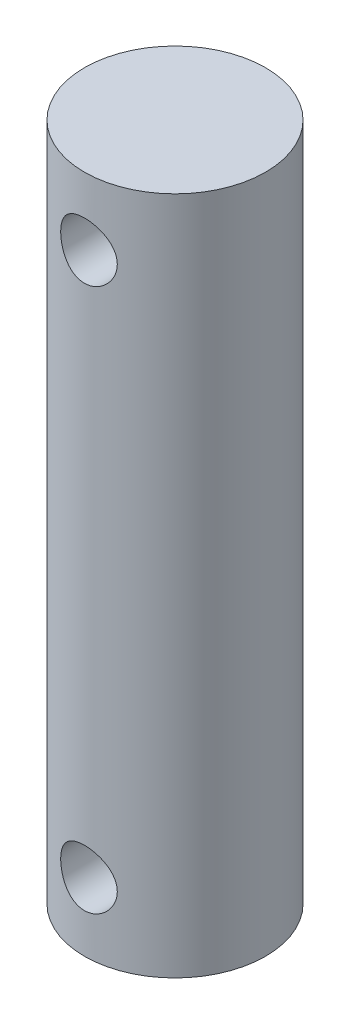
from build123d import *

# Parameters (mm, degrees)
PIN_PROFILE_16_R       = 8
PIN_BODY_16X60_DEPTH   = 30
CROSS_HOLES_DEPTH      = 33.062439084
CROSS_HOLES_DEPTH_BACK = 33.062439084
CROSS_HOLE_PROFILE_R   = 2.5


with BuildPart() as part:
    # Pin Profile Ø16 → Pin Body Ø16x60 (new, symmetric)
    with BuildSketch(Plane(origin=(0, 0, 0), x_dir=(1, 0, 0), z_dir=(0, 1, 0))):
        with Locations(Location((0, 0, 0), (0, 0, 270))):
            Circle(PIN_PROFILE_16_R)
    extrude(amount=PIN_BODY_16X60_DEPTH, both=True)

    # Cross Hole Profile → Cross Holes (cut, two sides: drawn at the far end of the back side and taken through both)
    with BuildSketch(Plane.XY.offset(-CROSS_HOLES_DEPTH_BACK)):
        with Locations(Location((0, 24, 0), (0, 0, 89.99999999))):
            Circle(CROSS_HOLE_PROFILE_R)
        with Locations(Location((0, -24, 0), (0, 0, 89.99999999))):
            Circle(CROSS_HOLE_PROFILE_R)
    extrude(amount=CROSS_HOLES_DEPTH + CROSS_HOLES_DEPTH_BACK, mode=Mode.SUBTRACT)


solid = part.part
